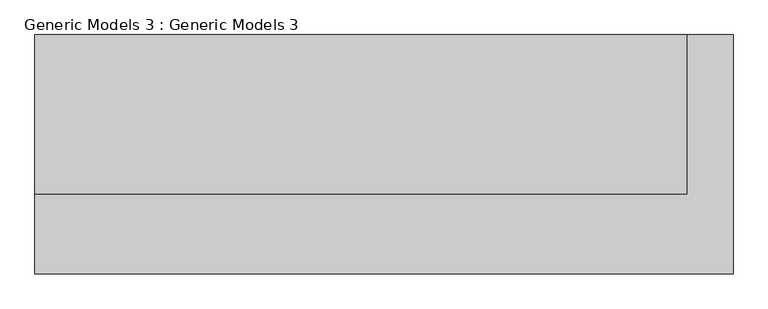
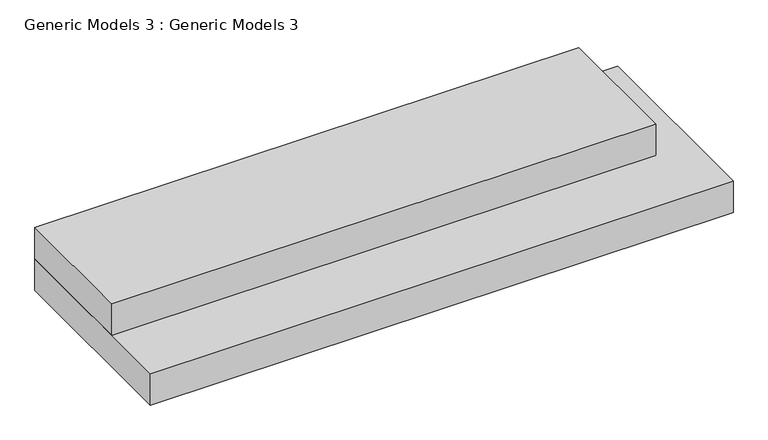
"""IFC4 building model written with IfcOpenShell, lengths in millimetres: proxy geometry, Generic Models 3 : Generic Models 3."""

from ifc_helpers import new_model, si_unit, frame, origin, origin_with_axes, place, context, project, spatial, polyline, outline, extrude, source, transform, mapped, element, save


def generic_models_3_generic_models_3_af6268f2(model_context):
    return source(origin(), model_context, "Body", "SweptSolid", [
        extrude(outline(polyline([(-12235.5371373, -4294.661407), (-14902.5371373, -4294.661407), (-14902.5371373, -3380.261407), (-12235.5371373, -3380.261407), (-12235.5371373, -4294.661407)])), origin_with_axes(), (0.0, 0.0, 1.0), 152.4),
        extrude(outline(polyline([(-12413.3371373, -3989.861407), (-14902.5371373, -3989.861407), (-14902.5371373, -3380.261407), (-12413.3371373, -3380.261407), (-12413.3371373, -3989.861407)])), frame((0.0, 0.0, 152.4), z_axis=(0.0, 0.0, 1.0), x_axis=(1.0, 0.0, 0.0)), (0.0, 0.0, 1.0), 152.4),
    ])


if __name__ == "__main__":
    model = new_model("IFC4")
    model_context = context("Model", 3, world=origin())
    ifc_project = project(units=[si_unit("LENGTHUNIT", "METRE", prefix="MILLI")], contexts=[model_context])
    site = spatial("IfcSite", under=ifc_project)
    building = spatial("IfcBuilding", under=site)
    placement = place(None, origin())
    generic_models_3_generic_models_3_shape = generic_models_3_generic_models_3_af6268f2(model_context)
    element("IfcBuildingElementProxy", 1, Name="Generic Models 3 : Generic Models 3", ObjectType="Generic Models 3 : Generic Models 3", at=placement, inside=building, context=model_context, shape_type="MappedRepresentation", body=[
        mapped(generic_models_3_generic_models_3_shape, transform((0.0, 0.0, 0.0), x_axis=(1.0, 0.0, 0.0), y_axis=(0.0, 1.0, 0.0), z_axis=(0.0, 0.0, 1.0))),
    ])
    save(model, "model.ifc")
